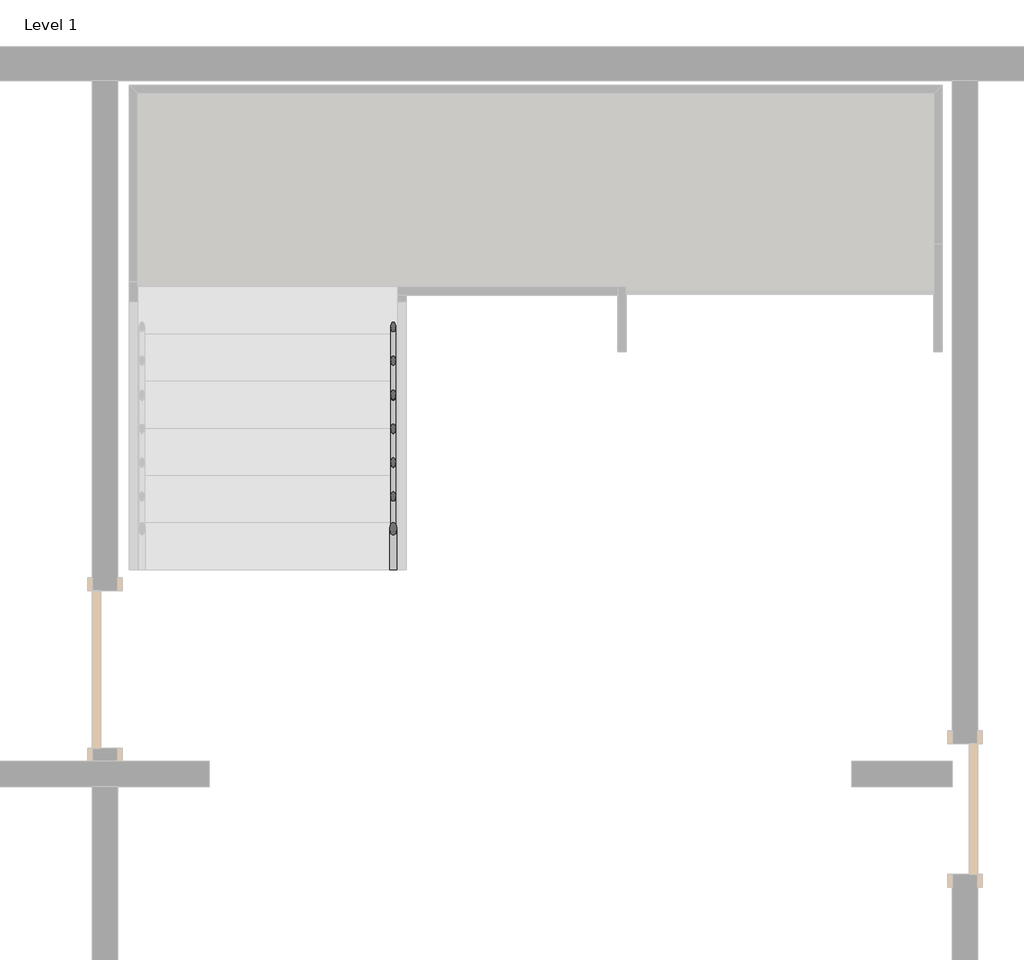
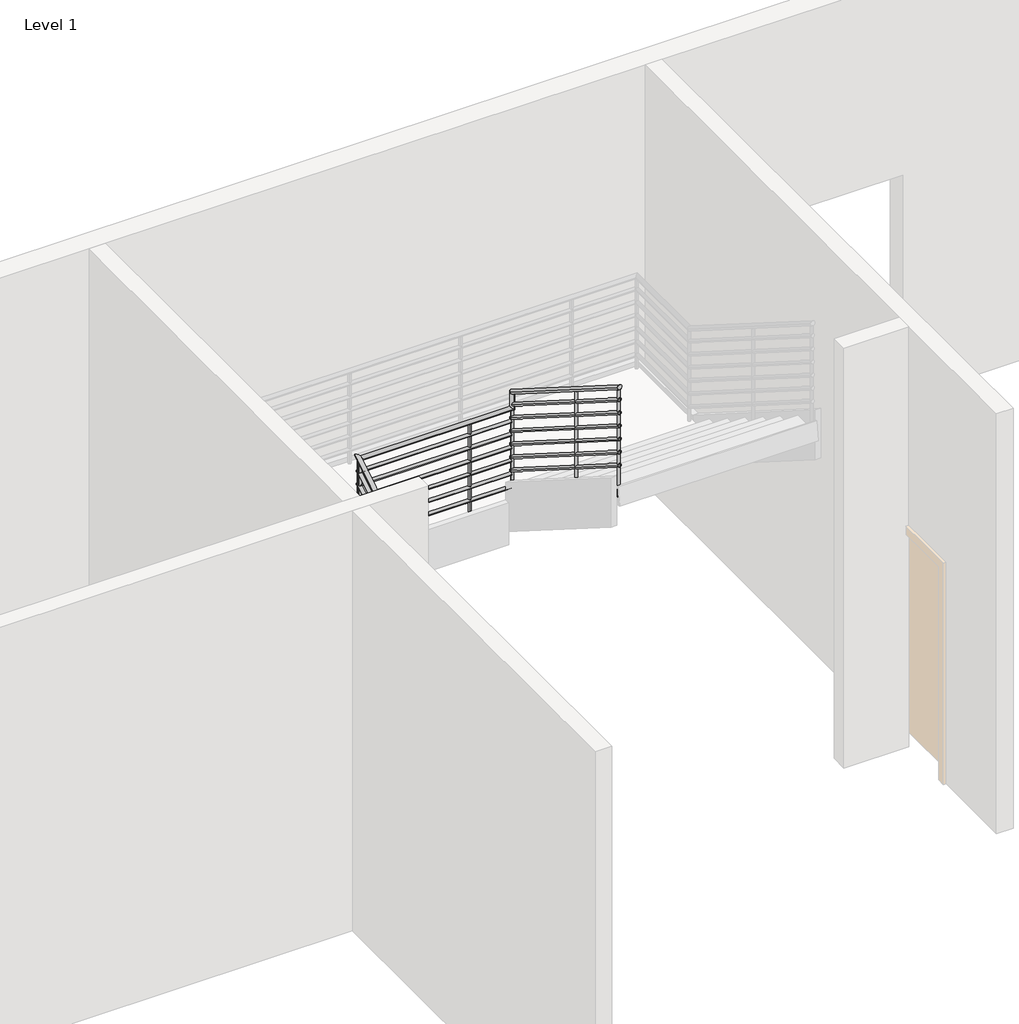
# One storey, part 2 of 3: 1 railing.
"""IFC4 building model written with IfcOpenShell, lengths in millimetres."""

from ifc_helpers import new_model, si_unit, point, frame, frame_2d, origin, place, context, project, spatial, circle_curve, ellipse_curve, trimmed, segment, composite_curve, outline, extrude, element, save
from ifc_brep_helpers import plane_surface, cylinder_surface, advanced_brep

model = new_model("IFC4")

# Units and contexts
model_context = context("Model", 3, world=origin())
ifc_project = project(units=[si_unit("LENGTHUNIT", "METRE", prefix="MILLI")], contexts=[model_context])

# Site, building, storey
site = spatial("IfcSite", under=ifc_project)
building = spatial("IfcBuilding", under=site)
storey = spatial("IfcBuildingStorey", under=building, Name="Level 1", Elevation=0.0)

# Railing
placement = place(None, origin())
element("IfcRailing", 1, ObjectType="900mm Pipe", at=placement, inside=storey, context=model_context, shape_type="SolidModel", body=[
    advanced_brep(
    [(-872.0164824, 8742.1981148, 1050.2491997), (-912.0164824, 8742.1981148, 1050.2491997), (-872.0164824, 10411.384603, 2105.861208), (-912.0164824, 10445.1914522, 2127.2410336)],
    [
        (0, 1, ellipse_curve(frame((-892.0164824, 8742.1981148, 1050.2491997), z_axis=(0.0, -1.0, 0.0), x_axis=(0.0, 0.0, -1.0)), 23.6638438, 20.0)),
        (1, 0, ellipse_curve(frame((-892.0164824, 8742.1981148, 1050.2491997), z_axis=(0.0, -1.0, 0.0), x_axis=(0.0, 0.0, -1.0)), 23.6638438, 20.0)),
        (2, 3, ellipse_curve(frame((-892.0164824, 10428.2880276, 2116.5511208), z_axis=(0.7071067811865487, 0.59762630898534, 0.3779454918484379), x_axis=(0.7071067811865467, -0.5976263089853422, -0.3779454918484378)), 28.2842712, 20.0)),
        (3, 2, ellipse_curve(frame((-892.0164824, 10428.2880276, 2116.5511208), z_axis=(0.7071067811865487, 0.59762630898534, 0.3779454918484379), x_axis=(0.7071067811865467, -0.5976263089853422, -0.3779454918484378)), 28.2842712, 20.0)),
        (0, 2),
        (3, 1),
    ],
    [
        plane_surface(frame((-892.0164824, 8742.1981148, 1073.9130435), z_axis=(0.0, -1.0, 0.0), x_axis=(0.0, 0.0, 1.0))),
        plane_surface(frame((-892.0164824, 10417.5981148, 2133.4545455), z_axis=(0.7071067811865486, 0.5976263089853399, 0.3779454918484378), x_axis=(0.7071067811865465, -0.5976263089853416, -0.3779454918484389))),
        cylinder_surface(frame((-892.0164824, 8752.8880276, 1057.0096189), z_axis=(0.0, -0.8451712313980433, -0.5344956404098309), x_axis=(-1.0, 0.0, 0.0)), 20.0),
    ],
    [
        (0, [[1, 2]]),
        (1, [[3, 4]]),
        (2, [[-1, 5, -4, 6]]),
        (2, [[-2, -6, -3, -5]]),
    ],
),
    advanced_brep(
    [(-864.423145, 10397.5981148, 2097.3913043), (-898.2299942, 10437.5981148, 2097.3913043), (491.6714992, 10397.5981148, 2097.3913043), (491.6714992, 10437.5981148, 2097.3913043)],
    [
        (0, 1, ellipse_curve(frame((-881.3265696, 10417.5981148, 2097.3913043), z_axis=(-0.7071067811865487, -0.59762630898534, -0.3779454918484379), x_axis=(-0.7071067811865464, 0.5976263089853424, 0.377945491848438)), 28.2842712, 20.0)),
        (1, 0, ellipse_curve(frame((-881.3265696, 10417.5981148, 2097.3913043), z_axis=(-0.7071067811865487, -0.59762630898534, -0.3779454918484379), x_axis=(-0.7071067811865464, 0.5976263089853424, 0.377945491848438)), 28.2842712, 20.0)),
        (2, 3, ellipse_curve(frame((491.6714992, 10417.5981148, 2097.3913043), z_axis=(0.7071067811865479, 0.0, 0.7071067811865471), x_axis=(-0.7071067811865471, 0.0, 0.7071067811865479)), 28.2842712, 20.0)),
        (3, 2, ellipse_curve(frame((491.6714992, 10417.5981148, 2097.3913043), z_axis=(0.7071067811865479, 0.0, 0.7071067811865471), x_axis=(-0.7071067811865471, 0.0, 0.7071067811865479)), 28.2842712, 20.0)),
        (0, 2),
        (3, 1),
    ],
    [
        plane_surface(frame((-892.0164824, 10417.5981148, 2117.3913043), z_axis=(-0.7071067811865486, -0.5976263089853399, -0.3779454918484378), x_axis=(0.7071067811865465, -0.5976263089853416, -0.3779454918484389))),
        plane_surface(frame((471.6714992, 10417.5981148, 2117.3913043), z_axis=(0.7071067811865479, 0.0, 0.7071067811865471), x_axis=(0.7071067811865471, 0.0, -0.7071067811865479))),
        cylinder_surface(frame((-892.0164824, 10417.5981148, 2097.3913043), z_axis=(-1.0, 0.0, 0.0), x_axis=(0.0, 1.0, 0.0)), 20.0),
    ],
    [
        (0, [[1, 2]]),
        (1, [[3, 4]]),
        (2, [[-1, 5, -4, 6]]),
        (2, [[-2, -6, -3, -5]]),
    ],
),
    advanced_brep(
    [(491.6714992, 10397.5981148, 2097.3913043), (491.6714992, 10437.5981148, 2097.3913043), (491.6714992, 10397.5981148, 2240.5616405), (491.6714992, 10437.5981148, 2262.5928854)],
    [
        (0, 1, ellipse_curve(frame((491.6714992, 10417.5981148, 2097.3913043), z_axis=(-0.7071067811865479, 0.0, -0.7071067811865471), x_axis=(0.707106781186547, 0.0, -0.707106781186548)), 28.2842712, 20.0)),
        (1, 0, ellipse_curve(frame((491.6714992, 10417.5981148, 2097.3913043), z_axis=(-0.7071067811865479, 0.0, -0.7071067811865471), x_axis=(0.707106781186547, 0.0, -0.707106781186548)), 28.2842712, 20.0)),
        (2, 3, ellipse_curve(frame((491.6714992, 10417.5981148, 2251.5772629), z_axis=(0.0, -0.48244396544581747, 0.8759268349610685), x_axis=(0.0, -0.8759268349610686, -0.4824439654458175)), 22.8329573, 20.0)),
        (3, 2, ellipse_curve(frame((491.6714992, 10417.5981148, 2251.5772629), z_axis=(0.0, -0.48244396544581747, 0.8759268349610685), x_axis=(0.0, -0.8759268349610686, -0.4824439654458175)), 22.8329573, 20.0)),
        (0, 2),
        (3, 1),
    ],
    [
        plane_surface(frame((491.6714992, 10417.5981148, 2097.3913043), z_axis=(-0.7071067811865479, 0.0, -0.7071067811865471), x_axis=(0.7071067811865471, 0.0, -0.7071067811865479))),
        plane_surface(frame((491.6714992, 10417.5981148, 2251.5772629), z_axis=(0.0, -0.48244396544581747, 0.8759268349610685), x_axis=(1.0, 0.0, 0.0))),
        cylinder_surface(frame((491.6714992, 10417.5981148, 2097.3913043), z_axis=(0.0, 0.0, -1.0), x_axis=(0.0, 1.0, 0.0)), 20.0),
    ],
    [
        (0, [[1, 2]]),
        (1, [[3, 4]]),
        (2, [[-1, 5, -4, 6]]),
        (2, [[-2, -6, -3, -5]]),
    ],
),
    advanced_brep(
    [(471.6714992, 10417.5981148, 2251.5772629), (511.6714992, 10417.5981148, 2251.5772629), (471.6714992, 8742.1981148, 3311.1187649), (511.6714992, 8742.1981148, 3311.1187649)],
    [
        (0, 1, ellipse_curve(frame((491.6714992, 10417.5981148, 2251.5772629), z_axis=(0.0, 0.48244396544581747, -0.8759268349610685), x_axis=(0.0, 0.8759268349610686, 0.4824439654458175)), 22.8329573, 20.0)),
        (1, 0, ellipse_curve(frame((491.6714992, 10417.5981148, 2251.5772629), z_axis=(0.0, 0.48244396544581747, -0.8759268349610685), x_axis=(0.0, 0.8759268349610686, 0.4824439654458175)), 22.8329573, 20.0)),
        (2, 3, ellipse_curve(frame((491.6714992, 8742.1981148, 3311.1187649), z_axis=(0.0, -1.0, 0.0), x_axis=(0.0, 0.0, -1.0)), 23.6638438, 20.0)),
        (3, 2, ellipse_curve(frame((491.6714992, 8742.1981148, 3311.1187649), z_axis=(0.0, -1.0, 0.0), x_axis=(0.0, 0.0, -1.0)), 23.6638438, 20.0)),
        (0, 2),
        (3, 1),
    ],
    [
        plane_surface(frame((491.6714992, 10437.5981148, 2262.5928854), z_axis=(0.0, 0.48244396544581747, -0.8759268349610685), x_axis=(1.0, 0.0, 0.0))),
        plane_surface(frame((491.6714992, 8742.1981148, 3334.7826087), z_axis=(0.0, -1.0, 0.0), x_axis=(0.0, 0.0, -1.0))),
        cylinder_surface(frame((491.6714992, 10426.908202, 2245.6894607), z_axis=(0.0, 0.845171231398044, -0.5344956404098298), x_axis=(1.0, 0.0, 0.0)), 20.0),
    ],
    [
        (0, [[1, 2]]),
        (1, [[3, 4]]),
        (2, [[-1, 5, -4, 6]]),
        (2, [[-2, -6, -3, -5]]),
    ],
),
    advanced_brep(
    [(-907.0164824, 8742.1981148, 931.1651606), (-877.0164824, 8742.1981148, 931.1651606), (-907.0164824, 10396.5432045, 1977.3913043), (-877.0164824, 10396.5432045, 1977.3913043), (-907.0164824, 10432.5981148, 1977.3913043), (-877.0164824, 10402.5981148, 1977.3913043), (476.6714992, 10432.5981148, 1977.3913043), (476.6714992, 10402.5981148, 1977.3913043)],
    [
        (0, 1, ellipse_curve(frame((-892.0164824, 8742.1981148, 931.1651606), z_axis=(0.0, -1.0, 0.0), x_axis=(0.0, 0.0, -1.0)), 17.7478828, 15.0)),
        (1, 0, ellipse_curve(frame((-892.0164824, 8742.1981148, 931.1651606), z_axis=(0.0, -1.0, 0.0), x_axis=(0.0, 0.0, -1.0)), 17.7478828, 15.0)),
        (0, 2),
        (2, 3, ellipse_curve(frame((-892.0164824, 10396.5432045, 1977.3913043), z_axis=(0.0, -0.9605132043335071, -0.2782344053149759), x_axis=(0.0, 0.27823440531497556, -0.9605132043335073)), 15.6166515, 15.0)),
        (3, 1),
        (3, 2, ellipse_curve(frame((-892.0164824, 10396.5432045, 1977.3913043), z_axis=(0.0, -0.9605132043335071, -0.2782344053149759), x_axis=(0.0, 0.27823440531497556, -0.9605132043335073)), 15.6166515, 15.0)),
        (2, 4),
        (4, 5, ellipse_curve(frame((-892.0164824, 10417.5981148, 1977.3913043), z_axis=(-0.7071067811865487, -0.7071067811865464, 0.0), x_axis=(0.7071067811865464, -0.7071067811865487, 0.0)), 21.2132034, 15.0)),
        (5, 3),
        (5, 4, ellipse_curve(frame((-892.0164824, 10417.5981148, 1977.3913043), z_axis=(-0.7071067811865487, -0.7071067811865464, 0.0), x_axis=(0.7071067811865464, -0.7071067811865487, 0.0)), 21.2132034, 15.0)),
        (6, 7, circle_curve(frame((476.6714992, 10417.5981148, 1977.3913043), z_axis=(1.0, 0.0, 0.0), x_axis=(0.0, -1.0, 0.0)), 15.0)),
        (7, 6, circle_curve(frame((476.6714992, 10417.5981148, 1977.3913043), z_axis=(1.0, 0.0, 0.0), x_axis=(0.0, -1.0, 0.0)), 15.0)),
        (4, 6),
        (7, 5),
    ],
    [
        plane_surface(frame((-892.0164824, 8742.1981148, 948.9130435), z_axis=(0.0, -1.0, 0.0), x_axis=(0.0, 0.0, 1.0))),
        cylinder_surface(frame((-892.0164824, 8750.2155494, 936.235475), z_axis=(0.0, -0.8451712313980434, -0.5344956404098308), x_axis=(1.0, 0.0, 0.0)), 15.0),
        cylinder_surface(frame((-892.0164824, 10392.1981148, 1977.3913043), z_axis=(0.0, -1.0, 0.0), x_axis=(1.0, 0.0, 0.0)), 15.0),
        plane_surface(frame((476.6714992, 10417.5981148, 1992.3913043), z_axis=(1.0, 0.0, 0.0), x_axis=(0.0, 1.0, 0.0))),
        cylinder_surface(frame((-892.0164824, 10417.5981148, 1977.3913043), z_axis=(-1.0, 0.0, 0.0), x_axis=(0.0, -1.0, 0.0)), 15.0),
    ],
    [
        (0, [[1, 2]]),
        (1, [[-1, 3, 4, 5]]),
        (1, [[-2, -5, 6, -3]]),
        (2, [[-4, 7, 8, 9]]),
        (2, [[-6, -9, 10, -7]]),
        (3, [[11, 12]]),
        (4, [[-8, 13, -12, 14]]),
        (4, [[-10, -14, -11, -13]]),
    ],
),
    advanced_brep(
    [(506.6714992, 10432.5981148, 2123.0070579), (476.6714992, 10432.5981148, 2123.0070579), (506.6714992, 8742.1981148, 3192.0347258), (476.6714992, 8742.1981148, 3192.0347258)],
    [
        (0, 1, ellipse_curve(frame((491.6714992, 10432.5981148, 2123.0070579), z_axis=(0.0, 1.0, 0.0), x_axis=(0.0, 0.0, -1.0)), 17.7478828, 15.0)),
        (1, 0, ellipse_curve(frame((491.6714992, 10432.5981148, 2123.0070579), z_axis=(0.0, 1.0, 0.0), x_axis=(0.0, 0.0, -1.0)), 17.7478828, 15.0)),
        (2, 3, ellipse_curve(frame((491.6714992, 8742.1981148, 3192.0347258), z_axis=(0.0, -1.0, 0.0), x_axis=(0.0, 0.0, -1.0)), 17.7478828, 15.0)),
        (3, 2, ellipse_curve(frame((491.6714992, 8742.1981148, 3192.0347258), z_axis=(0.0, -1.0, 0.0), x_axis=(0.0, 0.0, -1.0)), 17.7478828, 15.0)),
        (0, 2),
        (3, 1),
    ],
    [
        plane_surface(frame((491.6714992, 10432.5981148, 2140.7549407), z_axis=(0.0, 1.0, 0.0), x_axis=(0.0, 0.0, -1.0))),
        plane_surface(frame((491.6714992, 8742.1981148, 3209.7826087), z_axis=(0.0, -1.0, 0.0), x_axis=(0.0, 0.0, -1.0))),
        cylinder_surface(frame((491.6714992, 10424.5806802, 2128.0773722), z_axis=(0.0, 0.845171231398044, -0.5344956404098298), x_axis=(-1.0, 0.0, 0.0)), 15.0),
    ],
    [
        (0, [[1, 2]]),
        (1, [[3, 4]]),
        (2, [[-1, 5, -4, 6]]),
        (2, [[-2, -6, -3, -5]]),
    ],
),
    advanced_brep(
    [(-907.0164824, 8742.1981148, 806.1651606), (-877.0164824, 8742.1981148, 806.1651606), (-907.0164824, 10396.5432045, 1852.3913043), (-877.0164824, 10396.5432045, 1852.3913043), (-907.0164824, 10432.5981148, 1852.3913043), (-877.0164824, 10402.5981148, 1852.3913043), (476.6714992, 10432.5981148, 1852.3913043), (476.6714992, 10402.5981148, 1852.3913043)],
    [
        (0, 1, ellipse_curve(frame((-892.0164824, 8742.1981148, 806.1651606), z_axis=(0.0, -1.0, 0.0), x_axis=(0.0, 0.0, -1.0)), 17.7478828, 15.0)),
        (1, 0, ellipse_curve(frame((-892.0164824, 8742.1981148, 806.1651606), z_axis=(0.0, -1.0, 0.0), x_axis=(0.0, 0.0, -1.0)), 17.7478828, 15.0)),
        (0, 2),
        (2, 3, ellipse_curve(frame((-892.0164824, 10396.5432045, 1852.3913043), z_axis=(0.0, -0.9605132043335071, -0.2782344053149759), x_axis=(0.0, 0.27823440531497556, -0.9605132043335073)), 15.6166515, 15.0)),
        (3, 1),
        (3, 2, ellipse_curve(frame((-892.0164824, 10396.5432045, 1852.3913043), z_axis=(0.0, -0.9605132043335071, -0.2782344053149759), x_axis=(0.0, 0.27823440531497556, -0.9605132043335073)), 15.6166515, 15.0)),
        (2, 4),
        (4, 5, ellipse_curve(frame((-892.0164824, 10417.5981148, 1852.3913043), z_axis=(-0.7071067811865487, -0.7071067811865464, 0.0), x_axis=(0.7071067811865464, -0.7071067811865487, 0.0)), 21.2132034, 15.0)),
        (5, 3),
        (5, 4, ellipse_curve(frame((-892.0164824, 10417.5981148, 1852.3913043), z_axis=(-0.7071067811865487, -0.7071067811865464, 0.0), x_axis=(0.7071067811865464, -0.7071067811865487, 0.0)), 21.2132034, 15.0)),
        (6, 7, circle_curve(frame((476.6714992, 10417.5981148, 1852.3913043), z_axis=(1.0, 0.0, 0.0), x_axis=(0.0, -1.0, 0.0)), 15.0)),
        (7, 6, circle_curve(frame((476.6714992, 10417.5981148, 1852.3913043), z_axis=(1.0, 0.0, 0.0), x_axis=(0.0, -1.0, 0.0)), 15.0)),
        (4, 6),
        (7, 5),
    ],
    [
        plane_surface(frame((-892.0164824, 8742.1981148, 823.9130435), z_axis=(0.0, -1.0, 0.0), x_axis=(0.0, 0.0, 1.0))),
        cylinder_surface(frame((-892.0164824, 8750.2155494, 811.235475), z_axis=(0.0, -0.8451712313980434, -0.5344956404098308), x_axis=(1.0, 0.0, 0.0)), 15.0),
        cylinder_surface(frame((-892.0164824, 10392.1981148, 1852.3913043), z_axis=(0.0, -1.0, 0.0), x_axis=(1.0, 0.0, 0.0)), 15.0),
        plane_surface(frame((476.6714992, 10417.5981148, 1867.3913043), z_axis=(1.0, 0.0, 0.0), x_axis=(0.0, 1.0, 0.0))),
        cylinder_surface(frame((-892.0164824, 10417.5981148, 1852.3913043), z_axis=(-1.0, 0.0, 0.0), x_axis=(0.0, -1.0, 0.0)), 15.0),
    ],
    [
        (0, [[1, 2]]),
        (1, [[-1, 3, 4, 5]]),
        (1, [[-2, -5, 6, -3]]),
        (2, [[-4, 7, 8, 9]]),
        (2, [[-6, -9, 10, -7]]),
        (3, [[11, 12]]),
        (4, [[-8, 13, -12, 14]]),
        (4, [[-10, -14, -11, -13]]),
    ],
),
    advanced_brep(
    [(506.6714992, 10432.5981148, 1998.0070579), (476.6714992, 10432.5981148, 1998.0070579), (506.6714992, 8742.1981148, 3067.0347258), (476.6714992, 8742.1981148, 3067.0347258)],
    [
        (0, 1, ellipse_curve(frame((491.6714992, 10432.5981148, 1998.0070579), z_axis=(0.0, 1.0, 0.0), x_axis=(0.0, 0.0, -1.0)), 17.7478828, 15.0)),
        (1, 0, ellipse_curve(frame((491.6714992, 10432.5981148, 1998.0070579), z_axis=(0.0, 1.0, 0.0), x_axis=(0.0, 0.0, -1.0)), 17.7478828, 15.0)),
        (2, 3, ellipse_curve(frame((491.6714992, 8742.1981148, 3067.0347258), z_axis=(0.0, -1.0, 0.0), x_axis=(0.0, 0.0, -1.0)), 17.7478828, 15.0)),
        (3, 2, ellipse_curve(frame((491.6714992, 8742.1981148, 3067.0347258), z_axis=(0.0, -1.0, 0.0), x_axis=(0.0, 0.0, -1.0)), 17.7478828, 15.0)),
        (0, 2),
        (3, 1),
    ],
    [
        plane_surface(frame((491.6714992, 10432.5981148, 2015.7549407), z_axis=(0.0, 1.0, 0.0), x_axis=(0.0, 0.0, -1.0))),
        plane_surface(frame((491.6714992, 8742.1981148, 3084.7826087), z_axis=(0.0, -1.0, 0.0), x_axis=(0.0, 0.0, -1.0))),
        cylinder_surface(frame((491.6714992, 10424.5806802, 2003.0773722), z_axis=(0.0, 0.845171231398044, -0.5344956404098297), x_axis=(-1.0, 0.0, 0.0)), 15.0),
    ],
    [
        (0, [[1, 2]]),
        (1, [[3, 4]]),
        (2, [[-1, 5, -4, 6]]),
        (2, [[-2, -6, -3, -5]]),
    ],
),
    advanced_brep(
    [(-907.0164824, 8742.1981148, 681.1651606), (-877.0164824, 8742.1981148, 681.1651606), (-907.0164824, 10396.5432045, 1727.3913043), (-877.0164824, 10396.5432045, 1727.3913043), (-907.0164824, 10432.5981148, 1727.3913043), (-877.0164824, 10402.5981148, 1727.3913043), (476.6714992, 10432.5981148, 1727.3913043), (476.6714992, 10402.5981148, 1727.3913043)],
    [
        (0, 1, ellipse_curve(frame((-892.0164824, 8742.1981148, 681.1651606), z_axis=(0.0, -1.0, 0.0), x_axis=(0.0, 0.0, -1.0)), 17.7478828, 15.0)),
        (1, 0, ellipse_curve(frame((-892.0164824, 8742.1981148, 681.1651606), z_axis=(0.0, -1.0, 0.0), x_axis=(0.0, 0.0, -1.0)), 17.7478828, 15.0)),
        (0, 2),
        (2, 3, ellipse_curve(frame((-892.0164824, 10396.5432045, 1727.3913043), z_axis=(0.0, -0.9605132043335071, -0.2782344053149759), x_axis=(0.0, 0.27823440531497556, -0.9605132043335073)), 15.6166515, 15.0)),
        (3, 1),
        (3, 2, ellipse_curve(frame((-892.0164824, 10396.5432045, 1727.3913043), z_axis=(0.0, -0.9605132043335071, -0.2782344053149759), x_axis=(0.0, 0.27823440531497556, -0.9605132043335073)), 15.6166515, 15.0)),
        (2, 4),
        (4, 5, ellipse_curve(frame((-892.0164824, 10417.5981148, 1727.3913043), z_axis=(-0.7071067811865487, -0.7071067811865464, 0.0), x_axis=(0.7071067811865464, -0.7071067811865487, 0.0)), 21.2132034, 15.0)),
        (5, 3),
        (5, 4, ellipse_curve(frame((-892.0164824, 10417.5981148, 1727.3913043), z_axis=(-0.7071067811865487, -0.7071067811865464, 0.0), x_axis=(0.7071067811865464, -0.7071067811865487, 0.0)), 21.2132034, 15.0)),
        (6, 7, circle_curve(frame((476.6714992, 10417.5981148, 1727.3913043), z_axis=(1.0, 0.0, 0.0), x_axis=(0.0, -1.0, 0.0)), 15.0)),
        (7, 6, circle_curve(frame((476.6714992, 10417.5981148, 1727.3913043), z_axis=(1.0, 0.0, 0.0), x_axis=(0.0, -1.0, 0.0)), 15.0)),
        (4, 6),
        (7, 5),
    ],
    [
        plane_surface(frame((-892.0164824, 8742.1981148, 698.9130435), z_axis=(0.0, -1.0, 0.0), x_axis=(0.0, 0.0, 1.0))),
        cylinder_surface(frame((-892.0164824, 8750.2155494, 686.235475), z_axis=(0.0, -0.8451712313980434, -0.5344956404098308), x_axis=(1.0, 0.0, 0.0)), 15.0),
        cylinder_surface(frame((-892.0164824, 10392.1981148, 1727.3913043), z_axis=(0.0, -1.0, 0.0), x_axis=(1.0, 0.0, 0.0)), 15.0),
        plane_surface(frame((476.6714992, 10417.5981148, 1742.3913043), z_axis=(1.0, 0.0, 0.0), x_axis=(0.0, 1.0, 0.0))),
        cylinder_surface(frame((-892.0164824, 10417.5981148, 1727.3913043), z_axis=(-1.0, 0.0, 0.0), x_axis=(0.0, -1.0, 0.0)), 15.0),
    ],
    [
        (0, [[1, 2]]),
        (1, [[-1, 3, 4, 5]]),
        (1, [[-2, -5, 6, -3]]),
        (2, [[-4, 7, 8, 9]]),
        (2, [[-6, -9, 10, -7]]),
        (3, [[11, 12]]),
        (4, [[-8, 13, -12, 14]]),
        (4, [[-10, -14, -11, -13]]),
    ],
),
    advanced_brep(
    [(506.6714992, 10432.5981148, 1873.0070579), (476.6714992, 10432.5981148, 1873.0070579), (506.6714992, 8742.1981148, 2942.0347258), (476.6714992, 8742.1981148, 2942.0347258)],
    [
        (0, 1, ellipse_curve(frame((491.6714992, 10432.5981148, 1873.0070579), z_axis=(0.0, 1.0, 0.0), x_axis=(0.0, 0.0, -1.0)), 17.7478828, 15.0)),
        (1, 0, ellipse_curve(frame((491.6714992, 10432.5981148, 1873.0070579), z_axis=(0.0, 1.0, 0.0), x_axis=(0.0, 0.0, -1.0)), 17.7478828, 15.0)),
        (2, 3, ellipse_curve(frame((491.6714992, 8742.1981148, 2942.0347258), z_axis=(0.0, -1.0, 0.0), x_axis=(0.0, 0.0, -1.0)), 17.7478828, 15.0)),
        (3, 2, ellipse_curve(frame((491.6714992, 8742.1981148, 2942.0347258), z_axis=(0.0, -1.0, 0.0), x_axis=(0.0, 0.0, -1.0)), 17.7478828, 15.0)),
        (0, 2),
        (3, 1),
    ],
    [
        plane_surface(frame((491.6714992, 10432.5981148, 1890.7549407), z_axis=(0.0, 1.0, 0.0), x_axis=(0.0, 0.0, -1.0))),
        plane_surface(frame((491.6714992, 8742.1981148, 2959.7826087), z_axis=(0.0, -1.0, 0.0), x_axis=(0.0, 0.0, -1.0))),
        cylinder_surface(frame((491.6714992, 10424.5806802, 1878.0773722), z_axis=(0.0, 0.8451712313980441, -0.5344956404098297), x_axis=(-1.0, 0.0, 0.0)), 15.0),
    ],
    [
        (0, [[1, 2]]),
        (1, [[3, 4]]),
        (2, [[-1, 5, -4, 6]]),
        (2, [[-2, -6, -3, -5]]),
    ],
),
    advanced_brep(
    [(-907.0164824, 8742.1981148, 556.1651606), (-877.0164824, 8742.1981148, 556.1651606), (-907.0164824, 10396.5432045, 1602.3913043), (-877.0164824, 10396.5432045, 1602.3913043), (-907.0164824, 10432.5981148, 1602.3913043), (-877.0164824, 10402.5981148, 1602.3913043), (476.6714992, 10432.5981148, 1602.3913043), (476.6714992, 10402.5981148, 1602.3913043)],
    [
        (0, 1, ellipse_curve(frame((-892.0164824, 8742.1981148, 556.1651606), z_axis=(0.0, -1.0, 0.0), x_axis=(0.0, 0.0, -1.0)), 17.7478828, 15.0)),
        (1, 0, ellipse_curve(frame((-892.0164824, 8742.1981148, 556.1651606), z_axis=(0.0, -1.0, 0.0), x_axis=(0.0, 0.0, -1.0)), 17.7478828, 15.0)),
        (0, 2),
        (2, 3, ellipse_curve(frame((-892.0164824, 10396.5432045, 1602.3913043), z_axis=(0.0, -0.9605132043335071, -0.2782344053149759), x_axis=(0.0, 0.27823440531497556, -0.9605132043335073)), 15.6166515, 15.0)),
        (3, 1),
        (3, 2, ellipse_curve(frame((-892.0164824, 10396.5432045, 1602.3913043), z_axis=(0.0, -0.9605132043335071, -0.2782344053149759), x_axis=(0.0, 0.27823440531497556, -0.9605132043335073)), 15.6166515, 15.0)),
        (2, 4),
        (4, 5, ellipse_curve(frame((-892.0164824, 10417.5981148, 1602.3913043), z_axis=(-0.7071067811865487, -0.7071067811865464, 0.0), x_axis=(0.7071067811865464, -0.7071067811865487, 0.0)), 21.2132034, 15.0)),
        (5, 3),
        (5, 4, ellipse_curve(frame((-892.0164824, 10417.5981148, 1602.3913043), z_axis=(-0.7071067811865487, -0.7071067811865464, 0.0), x_axis=(0.7071067811865464, -0.7071067811865487, 0.0)), 21.2132034, 15.0)),
        (6, 7, circle_curve(frame((476.6714992, 10417.5981148, 1602.3913043), z_axis=(1.0, 0.0, 0.0), x_axis=(0.0, -1.0, 0.0)), 15.0)),
        (7, 6, circle_curve(frame((476.6714992, 10417.5981148, 1602.3913043), z_axis=(1.0, 0.0, 0.0), x_axis=(0.0, -1.0, 0.0)), 15.0)),
        (4, 6),
        (7, 5),
    ],
    [
        plane_surface(frame((-892.0164824, 8742.1981148, 573.9130435), z_axis=(0.0, -1.0, 0.0), x_axis=(0.0, 0.0, 1.0))),
        cylinder_surface(frame((-892.0164824, 8750.2155494, 561.235475), z_axis=(0.0, -0.8451712313980434, -0.5344956404098308), x_axis=(1.0, 0.0, 0.0)), 15.0),
        cylinder_surface(frame((-892.0164824, 10392.1981148, 1602.3913043), z_axis=(0.0, -1.0, 0.0), x_axis=(1.0, 0.0, 0.0)), 15.0),
        plane_surface(frame((476.6714992, 10417.5981148, 1617.3913043), z_axis=(1.0, 0.0, 0.0), x_axis=(0.0, 1.0, 0.0))),
        cylinder_surface(frame((-892.0164824, 10417.5981148, 1602.3913043), z_axis=(-1.0, 0.0, 0.0), x_axis=(0.0, -1.0, 0.0)), 15.0),
    ],
    [
        (0, [[1, 2]]),
        (1, [[-1, 3, 4, 5]]),
        (1, [[-2, -5, 6, -3]]),
        (2, [[-4, 7, 8, 9]]),
        (2, [[-6, -9, 10, -7]]),
        (3, [[11, 12]]),
        (4, [[-8, 13, -12, 14]]),
        (4, [[-10, -14, -11, -13]]),
    ],
),
    advanced_brep(
    [(506.6714992, 10432.5981148, 1748.0070579), (476.6714992, 10432.5981148, 1748.0070579), (506.6714992, 8742.1981148, 2817.0347258), (476.6714992, 8742.1981148, 2817.0347258)],
    [
        (0, 1, ellipse_curve(frame((491.6714992, 10432.5981148, 1748.0070579), z_axis=(0.0, 1.0, 0.0), x_axis=(0.0, 0.0, -1.0)), 17.7478828, 15.0)),
        (1, 0, ellipse_curve(frame((491.6714992, 10432.5981148, 1748.0070579), z_axis=(0.0, 1.0, 0.0), x_axis=(0.0, 0.0, -1.0)), 17.7478828, 15.0)),
        (2, 3, ellipse_curve(frame((491.6714992, 8742.1981148, 2817.0347258), z_axis=(0.0, -1.0, 0.0), x_axis=(0.0, 0.0, -1.0)), 17.7478828, 15.0)),
        (3, 2, ellipse_curve(frame((491.6714992, 8742.1981148, 2817.0347258), z_axis=(0.0, -1.0, 0.0), x_axis=(0.0, 0.0, -1.0)), 17.7478828, 15.0)),
        (0, 2),
        (3, 1),
    ],
    [
        plane_surface(frame((491.6714992, 10432.5981148, 1765.7549407), z_axis=(0.0, 1.0, 0.0), x_axis=(0.0, 0.0, -1.0))),
        plane_surface(frame((491.6714992, 8742.1981148, 2834.7826087), z_axis=(0.0, -1.0, 0.0), x_axis=(0.0, 0.0, -1.0))),
        cylinder_surface(frame((491.6714992, 10424.5806802, 1753.0773722), z_axis=(0.0, 0.845171231398044, -0.5344956404098297), x_axis=(-1.0, 0.0, 0.0)), 15.0),
    ],
    [
        (0, [[1, 2]]),
        (1, [[3, 4]]),
        (2, [[-1, 5, -4, 6]]),
        (2, [[-2, -6, -3, -5]]),
    ],
),
    advanced_brep(
    [(-907.0164824, 8742.1981148, 431.1651606), (-877.0164824, 8742.1981148, 431.1651606), (-907.0164824, 10396.5432045, 1477.3913043), (-877.0164824, 10396.5432045, 1477.3913043), (-907.0164824, 10432.5981148, 1477.3913043), (-877.0164824, 10402.5981148, 1477.3913043), (476.6714992, 10432.5981148, 1477.3913043), (476.6714992, 10402.5981148, 1477.3913043)],
    [
        (0, 1, ellipse_curve(frame((-892.0164824, 8742.1981148, 431.1651606), z_axis=(0.0, -1.0, 0.0), x_axis=(0.0, 0.0, -1.0)), 17.7478828, 15.0)),
        (1, 0, ellipse_curve(frame((-892.0164824, 8742.1981148, 431.1651606), z_axis=(0.0, -1.0, 0.0), x_axis=(0.0, 0.0, -1.0)), 17.7478828, 15.0)),
        (0, 2),
        (2, 3, ellipse_curve(frame((-892.0164824, 10396.5432045, 1477.3913043), z_axis=(0.0, -0.9605132043335071, -0.2782344053149759), x_axis=(0.0, 0.27823440531497556, -0.9605132043335073)), 15.6166515, 15.0)),
        (3, 1),
        (3, 2, ellipse_curve(frame((-892.0164824, 10396.5432045, 1477.3913043), z_axis=(0.0, -0.9605132043335071, -0.2782344053149759), x_axis=(0.0, 0.27823440531497556, -0.9605132043335073)), 15.6166515, 15.0)),
        (2, 4),
        (4, 5, ellipse_curve(frame((-892.0164824, 10417.5981148, 1477.3913043), z_axis=(-0.7071067811865487, -0.7071067811865464, 0.0), x_axis=(0.7071067811865464, -0.7071067811865487, 0.0)), 21.2132034, 15.0)),
        (5, 3),
        (5, 4, ellipse_curve(frame((-892.0164824, 10417.5981148, 1477.3913043), z_axis=(-0.7071067811865487, -0.7071067811865464, 0.0), x_axis=(0.7071067811865464, -0.7071067811865487, 0.0)), 21.2132034, 15.0)),
        (6, 7, circle_curve(frame((476.6714992, 10417.5981148, 1477.3913043), z_axis=(1.0, 0.0, 0.0), x_axis=(0.0, -1.0, 0.0)), 15.0)),
        (7, 6, circle_curve(frame((476.6714992, 10417.5981148, 1477.3913043), z_axis=(1.0, 0.0, 0.0), x_axis=(0.0, -1.0, 0.0)), 15.0)),
        (4, 6),
        (7, 5),
    ],
    [
        plane_surface(frame((-892.0164824, 8742.1981148, 448.9130435), z_axis=(0.0, -1.0, 0.0), x_axis=(0.0, 0.0, 1.0))),
        cylinder_surface(frame((-892.0164824, 8750.2155494, 436.235475), z_axis=(0.0, -0.8451712313980434, -0.5344956404098308), x_axis=(1.0, 0.0, 0.0)), 15.0),
        cylinder_surface(frame((-892.0164824, 10392.1981148, 1477.3913043), z_axis=(0.0, -1.0, 0.0), x_axis=(1.0, 0.0, 0.0)), 15.0),
        plane_surface(frame((476.6714992, 10417.5981148, 1492.3913043), z_axis=(1.0, 0.0, 0.0), x_axis=(0.0, 1.0, 0.0))),
        cylinder_surface(frame((-892.0164824, 10417.5981148, 1477.3913043), z_axis=(-1.0, 0.0, 0.0), x_axis=(0.0, -1.0, 0.0)), 15.0),
    ],
    [
        (0, [[1, 2]]),
        (1, [[-1, 3, 4, 5]]),
        (1, [[-2, -5, 6, -3]]),
        (2, [[-4, 7, 8, 9]]),
        (2, [[-6, -9, 10, -7]]),
        (3, [[11, 12]]),
        (4, [[-8, 13, -12, 14]]),
        (4, [[-10, -14, -11, -13]]),
    ],
),
    advanced_brep(
    [(506.6714992, 10432.5981148, 1623.0070579), (476.6714992, 10432.5981148, 1623.0070579), (506.6714992, 8742.1981148, 2692.0347258), (476.6714992, 8742.1981148, 2692.0347258)],
    [
        (0, 1, ellipse_curve(frame((491.6714992, 10432.5981148, 1623.0070579), z_axis=(0.0, 1.0, 0.0), x_axis=(0.0, 0.0, -1.0)), 17.7478828, 15.0)),
        (1, 0, ellipse_curve(frame((491.6714992, 10432.5981148, 1623.0070579), z_axis=(0.0, 1.0, 0.0), x_axis=(0.0, 0.0, -1.0)), 17.7478828, 15.0)),
        (2, 3, ellipse_curve(frame((491.6714992, 8742.1981148, 2692.0347258), z_axis=(0.0, -1.0, 0.0), x_axis=(0.0, 0.0, -1.0)), 17.7478828, 15.0)),
        (3, 2, ellipse_curve(frame((491.6714992, 8742.1981148, 2692.0347258), z_axis=(0.0, -1.0, 0.0), x_axis=(0.0, 0.0, -1.0)), 17.7478828, 15.0)),
        (0, 2),
        (3, 1),
    ],
    [
        plane_surface(frame((491.6714992, 10432.5981148, 1640.7549407), z_axis=(0.0, 1.0, 0.0), x_axis=(0.0, 0.0, -1.0))),
        plane_surface(frame((491.6714992, 8742.1981148, 2709.7826087), z_axis=(0.0, -1.0, 0.0), x_axis=(0.0, 0.0, -1.0))),
        cylinder_surface(frame((491.6714992, 10424.5806802, 1628.0773722), z_axis=(0.0, 0.845171231398044, -0.5344956404098298), x_axis=(-1.0, 0.0, 0.0)), 15.0),
    ],
    [
        (0, [[1, 2]]),
        (1, [[3, 4]]),
        (2, [[-1, 5, -4, 6]]),
        (2, [[-2, -6, -3, -5]]),
    ],
),
    advanced_brep(
    [(-907.0164824, 8742.1981148, 306.1651606), (-877.0164824, 8742.1981148, 306.1651606), (-907.0164824, 10396.5432045, 1352.3913043), (-877.0164824, 10396.5432045, 1352.3913043), (-907.0164824, 10432.5981148, 1352.3913043), (-877.0164824, 10402.5981148, 1352.3913043), (476.6714992, 10432.5981148, 1352.3913043), (476.6714992, 10402.5981148, 1352.3913043)],
    [
        (0, 1, ellipse_curve(frame((-892.0164824, 8742.1981148, 306.1651606), z_axis=(0.0, -1.0, 0.0), x_axis=(0.0, 0.0, -1.0)), 17.7478828, 15.0)),
        (1, 0, ellipse_curve(frame((-892.0164824, 8742.1981148, 306.1651606), z_axis=(0.0, -1.0, 0.0), x_axis=(0.0, 0.0, -1.0)), 17.7478828, 15.0)),
        (0, 2),
        (2, 3, ellipse_curve(frame((-892.0164824, 10396.5432045, 1352.3913043), z_axis=(0.0, -0.9605132043335071, -0.2782344053149759), x_axis=(0.0, 0.27823440531497556, -0.9605132043335073)), 15.6166515, 15.0)),
        (3, 1),
        (3, 2, ellipse_curve(frame((-892.0164824, 10396.5432045, 1352.3913043), z_axis=(0.0, -0.9605132043335071, -0.2782344053149759), x_axis=(0.0, 0.27823440531497556, -0.9605132043335073)), 15.6166515, 15.0)),
        (2, 4),
        (4, 5, ellipse_curve(frame((-892.0164824, 10417.5981148, 1352.3913043), z_axis=(-0.7071067811865487, -0.7071067811865464, 0.0), x_axis=(0.7071067811865464, -0.7071067811865487, 0.0)), 21.2132034, 15.0)),
        (5, 3),
        (5, 4, ellipse_curve(frame((-892.0164824, 10417.5981148, 1352.3913043), z_axis=(-0.7071067811865487, -0.7071067811865464, 0.0), x_axis=(0.7071067811865464, -0.7071067811865487, 0.0)), 21.2132034, 15.0)),
        (6, 7, circle_curve(frame((476.6714992, 10417.5981148, 1352.3913043), z_axis=(1.0, 0.0, 0.0), x_axis=(0.0, -1.0, 0.0)), 15.0)),
        (7, 6, circle_curve(frame((476.6714992, 10417.5981148, 1352.3913043), z_axis=(1.0, 0.0, 0.0), x_axis=(0.0, -1.0, 0.0)), 15.0)),
        (4, 6),
        (7, 5),
    ],
    [
        plane_surface(frame((-892.0164824, 8742.1981148, 323.9130435), z_axis=(0.0, -1.0, 0.0), x_axis=(0.0, 0.0, 1.0))),
        cylinder_surface(frame((-892.0164824, 8750.2155494, 311.235475), z_axis=(0.0, -0.8451712313980434, -0.5344956404098308), x_axis=(1.0, 0.0, 0.0)), 15.0),
        cylinder_surface(frame((-892.0164824, 10392.1981148, 1352.3913043), z_axis=(0.0, -1.0, 0.0), x_axis=(1.0, 0.0, 0.0)), 15.0),
        plane_surface(frame((476.6714992, 10417.5981148, 1367.3913043), z_axis=(1.0, 0.0, 0.0), x_axis=(0.0, 1.0, 0.0))),
        cylinder_surface(frame((-892.0164824, 10417.5981148, 1352.3913043), z_axis=(-1.0, 0.0, 0.0), x_axis=(0.0, -1.0, 0.0)), 15.0),
    ],
    [
        (0, [[1, 2]]),
        (1, [[-1, 3, 4, 5]]),
        (1, [[-2, -5, 6, -3]]),
        (2, [[-4, 7, 8, 9]]),
        (2, [[-6, -9, 10, -7]]),
        (3, [[11, 12]]),
        (4, [[-8, 13, -12, 14]]),
        (4, [[-10, -14, -11, -13]]),
    ],
),
    advanced_brep(
    [(506.6714992, 10432.5981148, 1498.0070579), (476.6714992, 10432.5981148, 1498.0070579), (506.6714992, 8742.1981148, 2567.0347258), (476.6714992, 8742.1981148, 2567.0347258)],
    [
        (0, 1, ellipse_curve(frame((491.6714992, 10432.5981148, 1498.0070579), z_axis=(0.0, 1.0, 0.0), x_axis=(0.0, 0.0, -1.0)), 17.7478828, 15.0)),
        (1, 0, ellipse_curve(frame((491.6714992, 10432.5981148, 1498.0070579), z_axis=(0.0, 1.0, 0.0), x_axis=(0.0, 0.0, -1.0)), 17.7478828, 15.0)),
        (2, 3, ellipse_curve(frame((491.6714992, 8742.1981148, 2567.0347258), z_axis=(0.0, -1.0, 0.0), x_axis=(0.0, 0.0, -1.0)), 17.7478828, 15.0)),
        (3, 2, ellipse_curve(frame((491.6714992, 8742.1981148, 2567.0347258), z_axis=(0.0, -1.0, 0.0), x_axis=(0.0, 0.0, -1.0)), 17.7478828, 15.0)),
        (0, 2),
        (3, 1),
    ],
    [
        plane_surface(frame((491.6714992, 10432.5981148, 1515.7549407), z_axis=(0.0, 1.0, 0.0), x_axis=(0.0, 0.0, -1.0))),
        plane_surface(frame((491.6714992, 8742.1981148, 2584.7826087), z_axis=(0.0, -1.0, 0.0), x_axis=(0.0, 0.0, -1.0))),
        cylinder_surface(frame((491.6714992, 10424.5806802, 1503.0773722), z_axis=(0.0, 0.845171231398044, -0.5344956404098297), x_axis=(-1.0, 0.0, 0.0)), 15.0),
    ],
    [
        (0, [[1, 2]]),
        (1, [[3, 4]]),
        (2, [[-1, 5, -4, 6]]),
        (2, [[-2, -6, -3, -5]]),
    ],
),
    advanced_brep(
    [(479.1714992, 9417.5981148, 2860.3244863), (479.1714992, 9417.5981148, 1913.0434783), (504.1714992, 9417.5981148, 1913.0434783), (504.1714992, 9417.5981148, 2860.3244863)],
    [
        (0, 1),
        (1, 2, circle_curve(frame((491.6714992, 9417.5981148, 1913.0434783), z_axis=(0.0, 0.0, 1.0), x_axis=(1.0, 0.0, 0.0)), 12.5)),
        (2, 3),
        (3, 0, ellipse_curve(frame((491.6714992, 9417.5981148, 2860.3244863), z_axis=(0.0, -0.5344956404098302, -0.8451712313980437), x_axis=(0.0, -0.8451712313980437, 0.53449564040983)), 14.7899024, 12.5)),
        (0, 3, ellipse_curve(frame((491.6714992, 9417.5981148, 2860.3244863), z_axis=(0.0, -0.5344956404098302, -0.8451712313980437), x_axis=(0.0, -0.8451712313980437, 0.53449564040983)), 14.7899024, 12.5)),
        (2, 1, circle_curve(frame((491.6714992, 9417.5981148, 1913.0434783), z_axis=(0.0, 0.0, 1.0), x_axis=(1.0, 0.0, 0.0)), 12.5)),
    ],
    [
        cylinder_surface(frame((491.6714992, 9417.5981148, 1813.0434783), z_axis=(0.0, 0.0, 1.0), x_axis=(1.0, 0.0, 0.0)), 12.5),
        plane_surface(frame((516.6714992, 9392.5981148, 2876.134763), z_axis=(0.0, 0.5344956404098302, 0.8451712313980437), x_axis=(-1.0, 0.0, 0.0))),
        plane_surface(frame((516.6714992, 9442.5981148, 1913.0434783), z_axis=(0.0, 0.0, -1.0), x_axis=(-1.0, 0.0, 0.0))),
    ],
    [
        (0, [[1, 2, 3, 4]]),
        (0, [[-1, 5, -3, 6]]),
        (1, [[-4, -5]]),
        (2, [[-2, -6]]),
    ],
),
    extrude(outline(composite_curve([segment(trimmed(circle_curve(frame_2d((107.9835176, 10417.5981148)), 12.5), [point((107.9835176, 10430.0981148))], [point((107.9835176, 10405.0981148))], False, "CARTESIAN"), True, "CONTINUOUS"), segment(trimmed(circle_curve(frame_2d((107.9835176, 10417.5981148)), 12.5), [point((107.9835176, 10405.0981148))], [point((107.9835176, 10430.0981148))], False, "CARTESIAN"), True, "CONTINUOUS")], self_intersect=False)), frame((0.0, 0.0, 1217.3913043), z_axis=(0.0, 0.0, 1.0), x_axis=(1.0, 0.0, 0.0)), (0.0, 0.0, 1.0), 860.0),
    advanced_brep(
    [(-879.5164824, 9742.1981148, 1658.9964231), (-879.5164824, 9742.1981148, 695.6521739), (-904.5164824, 9742.1981148, 695.6521739), (-904.5164824, 9742.1981148, 1658.9964231)],
    [
        (0, 1),
        (1, 2, circle_curve(frame((-892.0164824, 9742.1981148, 695.6521739), z_axis=(0.0, 0.0, 1.0), x_axis=(-1.0, 0.0, 0.0)), 12.5)),
        (2, 3),
        (3, 0, ellipse_curve(frame((-892.0164824, 9742.1981148, 1658.9964231), z_axis=(0.0, 0.5344956404098302, -0.8451712313980437), x_axis=(0.0, 0.8451712313980437, 0.53449564040983)), 14.7899024, 12.5)),
        (0, 3, ellipse_curve(frame((-892.0164824, 9742.1981148, 1658.9964231), z_axis=(0.0, 0.5344956404098302, -0.8451712313980437), x_axis=(0.0, 0.8451712313980437, 0.53449564040983)), 14.7899024, 12.5)),
        (2, 1, circle_curve(frame((-892.0164824, 9742.1981148, 695.6521739), z_axis=(0.0, 0.0, 1.0), x_axis=(-1.0, 0.0, 0.0)), 12.5)),
    ],
    [
        cylinder_surface(frame((-892.0164824, 9742.1981148, 595.6521739), z_axis=(0.0, 0.0, 1.0), x_axis=(-1.0, 0.0, 0.0)), 12.5),
        plane_surface(frame((-917.0164824, 9767.1981148, 1674.8066998), z_axis=(0.0, -0.5344956404098302, 0.8451712313980437), x_axis=(1.0, 0.0, 0.0))),
        plane_surface(frame((-917.0164824, 9717.1981148, 695.6521739), z_axis=(0.0, 0.0, -1.0), x_axis=(1.0, 0.0, 0.0))),
    ],
    [
        (0, [[1, 2, 3, 4]]),
        (0, [[-1, 5, -3, 6]]),
        (1, [[-4, -5]]),
        (2, [[-2, -6]]),
    ],
),
    extrude(outline(composite_curve([segment(trimmed(circle_curve(frame_2d((491.6714992, 10417.5981148)), 12.5), [point((504.1714992, 10417.5981148))], [point((479.1714992, 10417.5981148))], False, "CARTESIAN"), True, "CONTINUOUS"), segment(trimmed(circle_curve(frame_2d((491.6714992, 10417.5981148)), 12.5), [point((479.1714992, 10417.5981148))], [point((504.1714992, 10417.5981148))], False, "CARTESIAN"), True, "CONTINUOUS")], self_intersect=False)), frame((0.0, 0.0, 1217.3913043), z_axis=(0.0, 0.0, 1.0), x_axis=(1.0, 0.0, 0.0)), (0.0, 0.0, 1.0), 860.0),
    advanced_brep(
    [(-879.5164824, 10417.5981148, 2086.1268579), (-879.5164824, 10417.5981148, 1217.3913043), (-904.5164824, 10417.5981148, 1217.3913043), (-904.5164824, 10417.5981148, 2086.1268579)],
    [
        (0, 1),
        (1, 2, circle_curve(frame((-892.0164824, 10417.5981148, 1217.3913043), z_axis=(0.0, 0.0, 1.0), x_axis=(-1.0, 0.0, 0.0)), 12.5)),
        (2, 3),
        (3, 0, ellipse_curve(frame((-892.0164824, 10417.5981148, 2086.1268579), z_axis=(0.0, 0.5344956404098302, -0.8451712313980437), x_axis=(0.0, 0.8451712313980437, 0.53449564040983)), 14.7899024, 12.5)),
        (0, 3, ellipse_curve(frame((-892.0164824, 10417.5981148, 2086.1268579), z_axis=(0.0, 0.5344956404098302, -0.8451712313980437), x_axis=(0.0, 0.8451712313980437, 0.53449564040983)), 14.7899024, 12.5)),
        (2, 1, circle_curve(frame((-892.0164824, 10417.5981148, 1217.3913043), z_axis=(0.0, 0.0, 1.0), x_axis=(-1.0, 0.0, 0.0)), 12.5)),
    ],
    [
        cylinder_surface(frame((-892.0164824, 10417.5981148, 1117.3913043), z_axis=(0.0, 0.0, 1.0), x_axis=(-1.0, 0.0, 0.0)), 12.5),
        plane_surface(frame((-917.0164824, 10442.5981148, 2101.9371345), z_axis=(0.0, -0.5344956404098302, 0.8451712313980437), x_axis=(1.0, 0.0, 0.0))),
        plane_surface(frame((-917.0164824, 10392.5981148, 1217.3913043), z_axis=(0.0, 0.0, -1.0), x_axis=(1.0, 0.0, 0.0))),
    ],
    [
        (0, [[1, 2, 3, 4]]),
        (0, [[-1, 5, -3, 6]]),
        (1, [[-4, -5]]),
        (2, [[-2, -6]]),
    ],
),
    advanced_brep(
    [(-879.5164824, 10392.1981148, 2070.0636168), (-879.5164824, 10392.1981148, 1217.3913043), (-904.5164824, 10392.1981148, 1217.3913043), (-904.5164824, 10392.1981148, 2070.0636168)],
    [
        (0, 1),
        (1, 2, circle_curve(frame((-892.0164824, 10392.1981148, 1217.3913043), z_axis=(0.0, 0.0, 1.0), x_axis=(-1.0, 0.0, 0.0)), 12.5)),
        (2, 3),
        (3, 0, ellipse_curve(frame((-892.0164824, 10392.1981148, 2070.0636168), z_axis=(0.0, 0.5344956404098302, -0.8451712313980437), x_axis=(0.0, 0.8451712313980437, 0.53449564040983)), 14.7899024, 12.5)),
        (0, 3, ellipse_curve(frame((-892.0164824, 10392.1981148, 2070.0636168), z_axis=(0.0, 0.5344956404098302, -0.8451712313980437), x_axis=(0.0, 0.8451712313980437, 0.53449564040983)), 14.7899024, 12.5)),
        (2, 1, circle_curve(frame((-892.0164824, 10392.1981148, 1217.3913043), z_axis=(0.0, 0.0, 1.0), x_axis=(-1.0, 0.0, 0.0)), 12.5)),
    ],
    [
        cylinder_surface(frame((-892.0164824, 10392.1981148, 1117.3913043), z_axis=(0.0, 0.0, 1.0), x_axis=(-1.0, 0.0, 0.0)), 12.5),
        plane_surface(frame((-917.0164824, 10417.1981148, 2085.8738934), z_axis=(0.0, -0.5344956404098302, 0.8451712313980437), x_axis=(1.0, 0.0, 0.0))),
        plane_surface(frame((-917.0164824, 10367.1981148, 1217.3913043), z_axis=(0.0, 0.0, -1.0), x_axis=(1.0, 0.0, 0.0))),
    ],
    [
        (0, [[1, 2, 3, 4]]),
        (0, [[-1, 5, -3, 6]]),
        (1, [[-4, -5]]),
        (2, [[-2, -6]]),
    ],
),
    advanced_brep(
    [(479.1714992, 8754.6981148, 3279.5497828), (479.1714992, 8754.6981148, 2260.8695652), (504.1714992, 8754.6981148, 2260.8695652), (504.1714992, 8754.6981148, 3279.5497828)],
    [
        (0, 1),
        (1, 2, circle_curve(frame((491.6714992, 8754.6981148, 2260.8695652), z_axis=(0.0, 0.0, 1.0), x_axis=(1.0, 0.0, 0.0)), 12.5)),
        (2, 3),
        (3, 0, ellipse_curve(frame((491.6714992, 8754.6981148, 3279.5497828), z_axis=(0.0, -0.5344956404098302, -0.8451712313980437), x_axis=(0.0, -0.8451712313980437, 0.53449564040983)), 14.7899024, 12.5)),
        (0, 3, ellipse_curve(frame((491.6714992, 8754.6981148, 3279.5497828), z_axis=(0.0, -0.5344956404098302, -0.8451712313980437), x_axis=(0.0, -0.8451712313980437, 0.53449564040983)), 14.7899024, 12.5)),
        (2, 1, circle_curve(frame((491.6714992, 8754.6981148, 2260.8695652), z_axis=(0.0, 0.0, 1.0), x_axis=(1.0, 0.0, 0.0)), 12.5)),
    ],
    [
        cylinder_surface(frame((491.6714992, 8754.6981148, 2160.8695652), z_axis=(0.0, 0.0, 1.0), x_axis=(1.0, 0.0, 0.0)), 12.5),
        plane_surface(frame((516.6714992, 8729.6981148, 3295.3600594), z_axis=(0.0, 0.5344956404098302, 0.8451712313980437), x_axis=(-1.0, 0.0, 0.0))),
        plane_surface(frame((516.6714992, 8779.6981148, 2260.8695652), z_axis=(0.0, 0.0, -1.0), x_axis=(-1.0, 0.0, 0.0))),
    ],
    [
        (0, [[1, 2, 3, 4]]),
        (0, [[-1, 5, -3, 6]]),
        (1, [[-4, -5]]),
        (2, [[-2, -6]]),
    ],
),
    advanced_brep(
    [(-879.5164824, 8754.6981148, 1034.4904942), (-879.5164824, 8754.6981148, 173.9130435), (-904.5164824, 8754.6981148, 173.9130435), (-904.5164824, 8754.6981148, 1034.4904942)],
    [
        (0, 1),
        (1, 2, circle_curve(frame((-892.0164824, 8754.6981148, 173.9130435), z_axis=(0.0, 0.0, 1.0), x_axis=(-1.0, 0.0, 0.0)), 12.5)),
        (2, 3),
        (3, 0, ellipse_curve(frame((-892.0164824, 8754.6981148, 1034.4904942), z_axis=(0.0, 0.5344956404098302, -0.8451712313980437), x_axis=(0.0, 0.8451712313980437, 0.53449564040983)), 14.7899024, 12.5)),
        (0, 3, ellipse_curve(frame((-892.0164824, 8754.6981148, 1034.4904942), z_axis=(0.0, 0.5344956404098302, -0.8451712313980437), x_axis=(0.0, 0.8451712313980437, 0.53449564040983)), 14.7899024, 12.5)),
        (2, 1, circle_curve(frame((-892.0164824, 8754.6981148, 173.9130435), z_axis=(0.0, 0.0, 1.0), x_axis=(-1.0, 0.0, 0.0)), 12.5)),
    ],
    [
        cylinder_surface(frame((-892.0164824, 8754.6981148, 73.9130435), z_axis=(0.0, 0.0, 1.0), x_axis=(-1.0, 0.0, 0.0)), 12.5),
        plane_surface(frame((-917.0164824, 8779.6981148, 1050.3007709), z_axis=(0.0, -0.5344956404098302, 0.8451712313980437), x_axis=(1.0, 0.0, 0.0))),
        plane_surface(frame((-917.0164824, 8729.6981148, 173.9130435), z_axis=(0.0, 0.0, -1.0), x_axis=(1.0, 0.0, 0.0))),
    ],
    [
        (0, [[1, 2, 3, 4]]),
        (0, [[-1, 5, -3, 6]]),
        (1, [[-4, -5]]),
        (2, [[-2, -6]]),
    ],
),
])

save(model, "model.ifc")

# Revit data of these elements
# Type "900mm Pipe"
#   built-in parameter 1008612 = 0.019685 (stored number, unit not read)
#   built-in parameter 1008611 = 0.0984252 (stored number, unit not read)
#   built-in parameter 1008609 = 6.56168 (stored number, unit not read)
#   built-in parameter 1008604 = 0.19685 (stored number, unit not read)
#   built-in parameter 1008603 = 0.164042 (stored number, unit not read)
#   Railing Height = 900 mm
#   built-in parameter 1008630 = 2
#   built-in parameter 1008610 = 2
#   built-in parameter 1008605 = 1
#   built-in parameter 1008618 = M_Baluster - Round : 25mm
# Element 1 (IfcRailing, "900mm Pipe")
#   Phase Created = New Construction
